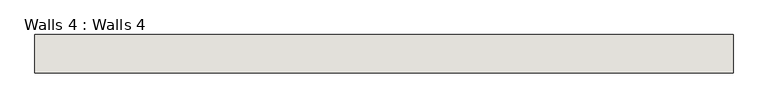
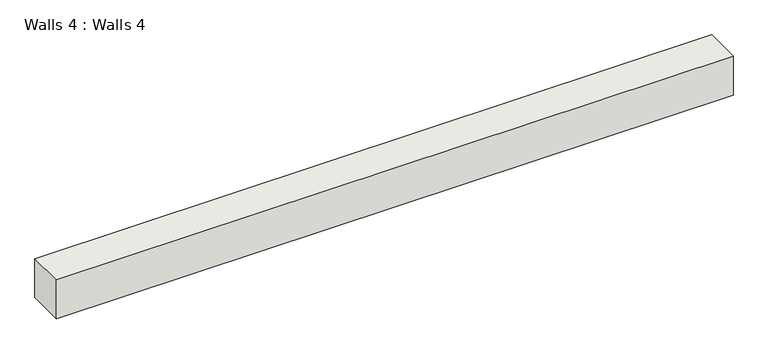
"""IFC4 building model written with IfcOpenShell, lengths in millimetres: wall geometry, Walls 4 : Walls 4."""

from ifc_helpers import new_model, si_unit, frame, origin, place, context, project, spatial, polyline, outline, extrude, source, transform, mapped, element, save


def walls_4_walls_4_2164e9f1(model_context):
    return source(origin(), model_context, "Body", "SweptSolid", [
        extrude(outline(polyline([(-6840.0943623, 5254.5756066), (-11863.1736868, 5254.5756066), (-11863.1736868, 5530.334124), (-6840.0943623, 5530.334124), (-6840.0943623, 5254.5756066)])), frame((0.0, 0.0, 3657.6), z_axis=(0.0, 0.0, 1.0), x_axis=(1.0, 0.0, 0.0)), (0.0, 0.0, 1.0), 304.8),
    ])


if __name__ == "__main__":
    model = new_model("IFC4")
    model_context = context("Model", 3, world=origin())
    ifc_project = project(units=[si_unit("LENGTHUNIT", "METRE", prefix="MILLI")], contexts=[model_context])
    site = spatial("IfcSite", under=ifc_project)
    building = spatial("IfcBuilding", under=site)
    placement = place(None, origin())
    walls_4_walls_4_shape = walls_4_walls_4_2164e9f1(model_context)
    element("IfcWall", 1, ObjectType="Walls 4 : Walls 4", at=placement, inside=building, context=model_context, shape_type="MappedRepresentation", body=[
        mapped(walls_4_walls_4_shape, transform((0.0, 0.0, 0.0), x_axis=(1.0, 0.0, 0.0), y_axis=(0.0, 1.0, 0.0), z_axis=(0.0, 0.0, 1.0))),
    ])
    save(model, "model.ifc")

# Revit data of these elements
# Element 1 (IfcWall, "Walls 4 : Walls 4")
#   Materials on its faces: "Default Wall"
# Materials
#   "Default Wall": colour RGB 128 128 128, transparency 0
